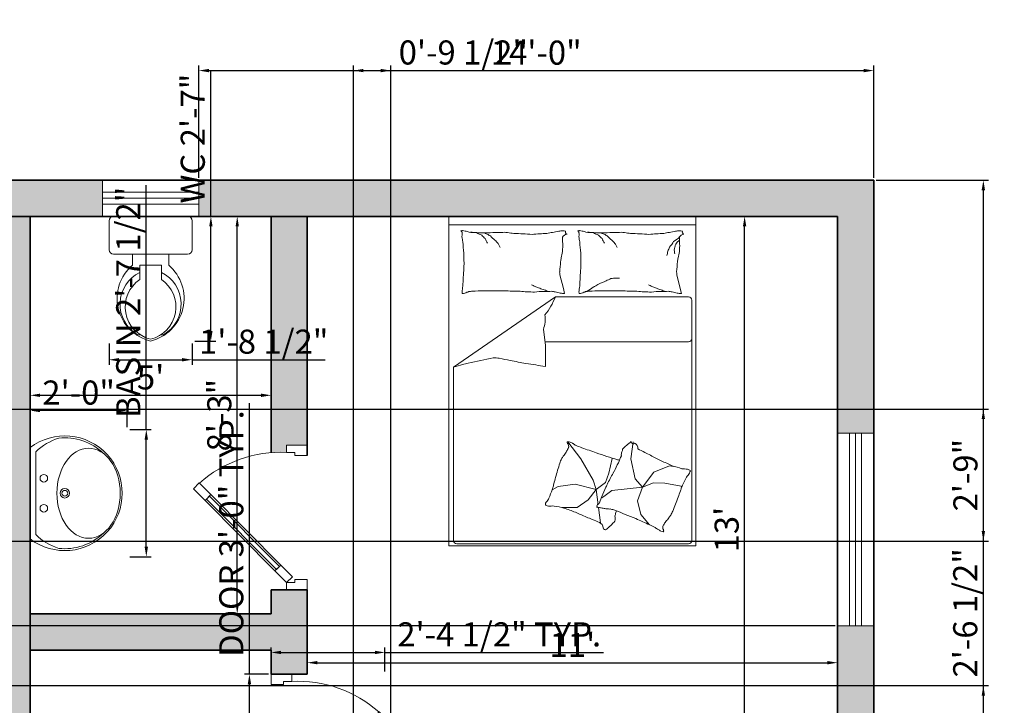
# Model space of a CAD drawing. Units: inches. Extents: x -40 to 424, y -33 to 568.
# Tile 8 of 8: x 171 to 417, y 397 to 568. Entities that reach past the tile are written whole.
import ezdxf

# ---------------------------------------------------------------- set-up
doc = ezdxf.new("R2010")
doc.units = ezdxf.units.IN
for name, color, linetype, lineweight in [('A-ANNO-DIMS', 7, 'Continuous', 18), ('A-DOOR', 7, 'Continuous', 18), ('A-FLOR-FIXT', 7, 'Continuous', 18), ('A-FURN', 7, 'Continuous', 18), ('A-GLAZ', 7, 'Continuous', 18), ('A-WALL-PATT', 30, 'Continuous', 13), ('wall', 7, 'Continuous', 35)]:
    doc.layers.add(name, color=color, linetype=linetype, lineweight=lineweight)
doc.styles.add('DIM_FONT', font='SIMPLEX.shx', dxfattribs={"width": 0.8})
doc.styles.get("Standard").update_dxf_attribs({"font": 'arial.ttf'})
doc.dimstyles.new('ISO-25', dxfattribs={"dimtxt": 6, "dimasz": 2.5, "dimexe": 1.25, "dimexo": 0.625, "dimtad": 1, "dimdec": 1, "dimlunit": 3, "dimtxsty": 'Standard', "dimcen": 2.5, "dimadec": 0, "dimazin": 0, "dimtfac": 1, "dimtdec": 1, "dimtmove": 0, "dimatfit": 3, "dimfxl": 1, "dimarcsym": 0})

# ---------------------------------------------------------------- blocks, each defined once
blk = doc.blocks.new('A$C3C032968')
for p, q in [((0, 0), (0, 100)), ((0, 100), (0, 0)), ((700, 0), (700, 100)), ((700, 0), (700, 100))]:
    blk.add_line(p, q)
for points in [[(517.5, 522.4), (460.7, 466.1), (432.5, 494.5), (489.3, 550.8)], [(120, 128), (460.7, 466.1), (432.5, 494.5), (91.8, 156.4)], [(112.9, 135.1), (453.6, 473.2), (439.5, 487.4), (98.8, 149.3)], [(63.2, 71.6), (120, 128), (91.8, 156.4), (35, 100)], [(35, 100), (0, 100), (0, 0), (50, 0), (50, 50), (50, 60), (35, 60)], [(665, 100), (665, 60), (650, 60), (650, 50), (650, 0), (700, 0), (700, 100)]]:
    blk.add_lwpolyline(points, close=True)
blk.add_arc((72.4, 128.7), 593.3, 357.2313, 41.4937)
blk = doc.blocks.new('A$C79B528CE')
for p, q in [((1.5, 2), (0, 2)), ((0, 2), (0, 0)), ((1.5, 0), (1.5, 2)), ((1.5, 1.9476), (0, 1.9476)), ((0.6954, 1.5617), (0.6748, 1.6443)), ((1.4047, 1.5617), (1.384, 1.6443)), ((0.7029, 1.5317), (0.6954, 1.5617)), ((1.4122, 1.5317), (1.4047, 1.5617)), ((0.6465, 1.5115), (0.0284, 1.0841)), ((0.6465, 1.5115), (1.4542, 1.5115)), ((1.4742, 1.4915), (1.4742, 0.0322)), ((0.574, 1.3138), (0.5876, 1.2184)), ((1.4542, 1.2389), (0.5847, 1.2389)), ((0.5876, 1.2184), (0.5859, 1.0883)), ((0.0284, 0.0322), (0.0284, 1.0841)), ((0.7224, 0.6316), (0.8016, 0.5276)), ((1.119, 0.6317), (1.1052, 0.5286)), ((0.8016, 0.5276), (0.8767, 0.3973)), ((0.9716, 0.4407), (0.9914, 0.5296)), ((1.1052, 0.5286), (1.131, 0.4065)), ((1.2446, 0.4478), (1.3392, 0.4856)), ((1.3392, 0.4856), (1.3632, 0.4822)), ((0.9518, 0.3834), (0.9716, 0.4407)), ((1.1757, 0.355), (1.2446, 0.4478)), ((0.6632, 0.3597), (0.6272, 0.3397)), ((0.766, 0.3736), (0.6632, 0.3597)), ((0.8945, 0.342), (0.766, 0.3736)), ((0.8767, 0.3973), (0.8945, 0.342)), ((0.8945, 0.342), (0.9518, 0.3834)), ((1.131, 0.4065), (1.1757, 0.355)), ((1.1757, 0.355), (1.2428, 0.3825)), ((1.2428, 0.3825), (1.3116, 0.379)), ((1.3116, 0.379), (1.4097, 0.3619)), ((1.4097, 0.3619), (1.413, 0.3554)), ((0.8945, 0.342), (0.8451, 0.2787)), ((0.8945, 0.342), (0.9063, 0.2478)), ((0.9297, 0.2995), (0.9119, 0.256)), ((0.9401, 0.3), (0.928, 0.2914)), ((0.9527, 0.3558), (0.9297, 0.2995)), ((0.99, 0.3361), (0.9401, 0.3)), ((1.1757, 0.355), (0.99, 0.3361)), ((1.1757, 0.355), (1.1448, 0.2725)), ((0.8451, 0.2787), (0.7799, 0.2313)), ((1.1448, 0.2725), (1.1654, 0.19)), ((0.7799, 0.2313), (0.687, 0.2313)), ((0.9081, 0.2331), (0.92, 0.1385)), ((1.1654, 0.19), (1.219, 0.1274)), ((1.4542, 0.0122), (0.0484, 0.0122)), ((0, 0), (1.5, 0))]:
    blk.add_line(p, q)
for centre, radius, start, end in [((0.0726, 1.9139), 0.00342, 291.7883, 340.43603), ((0.0739, 1.9378), 0.0251, 274.30254, 291.7883), ((0.098, 1.9393), 0.0289, 239.34875, 274.30254), ((0.6672, 2.0719), 0.1611, 270, 278.43719), ((0.7086, 2.0011), 0.0904, 258.72762, 270), ((0.7818, 1.9139), 0.00342, 291.7883, 340.43603), ((0.7831, 1.9378), 0.0251, 274.30254, 291.7883), ((0.8072, 1.9393), 0.0289, 239.34875, 274.30254), ((1.3765, 2.0719), 0.1611, 270, 278.43719), ((1.4178, 2.0011), 0.0904, 258.72762, 270), ((0.0743, 1.9085), 0.00232, 340.43603, 101.89306), ((0.0805, 1.9093), 0.00428, 201.9904, 281.89306), ((0.049, 1.8889), 0.0328, 338.57902, 8.13348), ((-0.1611, 1.8253), 0.246, 8.13348, 12.10946), ((0.0959, 1.8994), 0.0156, 158.57902, 201.9904), ((0.279, 1.8867), 0.1983, 187.6809, 192.10946), ((0.0952, 1.8568), 0.0539, 59.34875, 84.74081), ((0.0953, 1.0829), 0.8208, 84.74081, 88.09211), ((0.1612, 2.0005), 0.0992, 254.06476, 274.21588), ((0.2269, 1.9817), 0.0992, 233.91364, 254.06476), ((0.1856, 0.406), 1.4943, 88.09211, 90.57574), ((0.2797, 1.9449), 0.0992, 216.17665, 233.91364), ((0.323, 2.1075), 0.234, 242.76041, 249.13972), ((0.3154, 1.8961), 0.0992, 198.43965, 216.17665), ((0.3084, 1.0293), 0.8732, 90.57574, 94.80185), ((0.2874, 1.949), 0.0768, 231.61143, 242.76041), ((0.5234, 2.1633), 0.3916, 226.18849, 231.61143), ((0.4551, 1.9982), 0.2252, 219.03494, 226.18849), ((0.3125, 2.1919), 0.2897, 267.46141, 274.80185), ((0.3637, 2.0532), 0.1524, 259.81012, 267.46141), ((0.3008, 1.3747), 0.5293, 79.81012, 83.9133), ((0.3945, 0.8466), 1.049, 83.9133, 90), ((0.5954, 1.2129), 0.6827, 90, 97.54685), ((0.6611, 1.6625), 0.2422, 97.54685, 105.74398), ((0.5846, 2.2041), 0.3048, 278.43719, 285.74398), ((0.7204, 1.8579), 0.0342, 94.40021, 153.41948), ((1.1818, 1.8735), 0.4918, 180, 186.23236), ((0.7203, 1.9049), 0.0131, 153.41948, 258.72762), ((0.7836, 1.9085), 0.00232, 340.43603, 101.89306), ((0.7897, 1.9093), 0.00428, 201.9904, 281.89306), ((0.7582, 1.8889), 0.0328, 338.57902, 8.13348), ((0.5482, 1.8253), 0.246, 8.13348, 12.10946), ((0.8051, 1.8994), 0.0156, 158.57902, 201.9904), ((0.9883, 1.8867), 0.1983, 187.6809, 192.10946), ((0.8044, 1.8568), 0.0539, 59.34875, 84.74081), ((0.8046, 1.0829), 0.8208, 84.74081, 88.09211), ((0.8704, 2.0005), 0.0992, 254.06476, 274.21588), ((0.9361, 1.9817), 0.0992, 233.91364, 254.06476), ((0.8948, 0.406), 1.4943, 88.09211, 90.57574), ((0.989, 1.9449), 0.0992, 216.17665, 233.91364), ((1.0323, 2.1075), 0.234, 242.76041, 249.13972), ((1.0247, 1.8961), 0.0992, 198.43965, 216.17665), ((1.0177, 1.0293), 0.8732, 90.57574, 94.80185), ((0.9966, 1.949), 0.0768, 231.61143, 242.76041), ((1.2326, 2.1633), 0.3916, 226.18849, 231.61143), ((1.1643, 1.9982), 0.2252, 219.03494, 226.18849), ((1.0217, 2.1919), 0.2897, 267.46141, 274.80185), ((1.0729, 2.0532), 0.1524, 259.81012, 267.46141), ((1.0101, 1.3747), 0.5293, 79.81012, 83.9133), ((1.1037, 0.8466), 1.049, 83.9133, 90), ((1.3046, 1.2129), 0.6827, 90, 97.54685), ((1.3703, 1.6625), 0.2422, 97.54685, 105.74398), ((1.2938, 2.2041), 0.3048, 278.43719, 285.74398), ((1.3004, 1.9723), 0.1399, 297.20359, 314.90238), ((1.3333, 1.9167), 0.0899, 306.26407, 318.55709), ((1.4296, 1.8579), 0.0342, 94.40021, 153.41948), ((1.891, 1.8735), 0.4918, 180, 186.23236), ((1.4295, 1.9049), 0.0131, 153.41948, 258.72762), ((0.9966, 1.8987), 0.9131, 183.36875, 187.6809), ((0.3426, 1.8591), 0.0493, 208.31676, 219.03494), ((0.4886, 1.9062), 0.2002, 203.00277, 208.31676), ((0.8939, 1.7858), 0.204, 170.31563, 180), ((1.7058, 1.8987), 0.9131, 183.36875, 187.6809), ((1.0518, 1.8591), 0.0493, 208.31676, 219.03494), ((1.1978, 1.9062), 0.2002, 203.00277, 208.31676), ((1.2048, 1.8529), 0.1399, 332.60117, 343.48502), ((1.2401, 1.9123), 0.1399, 314.90238, 332.60117), ((1.3147, 1.8132), 0.0562, 341.2201, 0), ((1.2793, 1.7719), 0.0915, 0, 14.68511), ((1.18, 1.8895), 0.2056, 338.18508, 341.2201), ((1.2381, 1.8881), 0.1511, 334.64488, 338.18508), ((1.3389, 1.8667), 0.0526, 318.55709, 334.64488), ((1.6031, 1.7858), 0.204, 170.31563, 180), ((0.7702, 1.7573), 0.6787, 178.36691, 183.36875), ((0.3686, 1.792), 0.3171, 347.80162, 351.99495), ((1.552, 1.5994), 0.882, 167.80162, 170.31563), ((1.4794, 1.7573), 0.6787, 178.36691, 183.36875), ((1.1897, 1.8023), 0.1399, 343.48502, 354.36887), ((1.0778, 1.792), 0.3171, 347.80162, 351.99495), ((2.2613, 1.5994), 0.882, 167.80162, 170.31563), ((13.7013, 0.85), 13.6356, 176.49514, 176.94504), ((1.4559, 1.6447), 1.3652, 176.94504, 178.36691), ((0.0204, 1.7556), 0.6588, 351.99495, 357.33512), ((14.4105, 0.85), 13.6356, 176.49514, 176.94504), ((2.1651, 1.6447), 1.3652, 176.94504, 178.36691), ((0.7297, 1.7556), 0.6588, 351.99495, 357.33512), ((0.6071, 1.6474), 0.0677, 357.33512, 14.04519), ((0.7753, 2.0834), 0.5066, 290.67428, 294.32653), ((0.9799, 1.6796), 0.058, 274.08277, 290.67428), ((1.0172, 1.8969), 0.2721, 266.4448, 274.08277), ((1.3164, 1.6474), 0.0677, 357.33512, 14.04519), ((0.4014, 1.5209), 0.3212, 170.00164, 176.49514), ((0.2076, 0.9067), 0.7387, 64.68893, 66.51559), ((0.2508, 0.888), 0.7387, 66.51559, 68.34226), ((0.2995, 0.8688), 0.7387, 68.34226, 70.57202), ((0.3537, 0.8497), 0.7387, 70.57202, 72.80178), ((1.1107, 1.5209), 0.3212, 170.00164, 176.49514), ((0.4519, 2.1618), 0.7286, 302.13498, 305.82629), ((0.7388, 1.8508), 0.3126, 296.49848, 302.13498), ((0.3151, 2.8912), 1.4323, 294.32653, 296.49848), ((0.9169, 0.9067), 0.7387, 64.68893, 66.51559), ((0.9601, 0.888), 0.7387, 66.51559, 68.34226), ((1.0087, 0.8688), 0.7387, 68.34226, 70.57202), ((1.0629, 0.8497), 0.7387, 70.57202, 72.80178), ((0.0623, 1.535), 0.0193, 350.00164, 16.69777), ((0.0815, 1.5304), 0.00132, 16.69777, 97.12039), ((0.1072, 1.4467), 0.0875, 97.12039, 106.22115), ((0.1315, 1.4654), 0.0767, 106.22115, 117.28412), ((0.1, 1.5832), 0.0453, 282.86904, 297.28412), ((0.1117, 1.6885), 0.1459, 273.57397, 282.86904), ((0.1384, 2.7103), 1.164, 270.28654, 273.57397), ((0.3078, 7.2662), 5.7185, 269.02962, 270.28654), ((0.4895, 4.9065), 3.3622, 267.39037, 269.02962), ((0.5304, 2.7573), 1.2165, 265.38242, 267.39037), ((0.4077, 0.139), 1.4048, 85.38242, 87.25094), ((0.5669, 1.3138), 0.2301, 87.25094, 101.55856), ((0.5943, 1.6886), 0.1459, 263.56595, 281.55856), ((0.2944, 1.6407), 0.3751, 320.35546, 339.85116), ((0.6593, 1.6599), 0.1197, 252.61359, 263.56595), ((0.608, 1.3144), 0.2297, 72.61359, 80.5159), ((0.6574, 1.2635), 0.2708, 80.5159, 85.91706), ((0.7029, 1.5308), 0.000917, 85.91706, 194.04494), ((0.7716, 1.535), 0.0193, 350.00164, 16.69777), ((0.7908, 1.5304), 0.00132, 16.69777, 97.12039), ((0.8165, 1.4467), 0.0875, 97.12039, 106.22115), ((0.8408, 1.4654), 0.0767, 106.22115, 117.28412), ((0.8093, 1.5832), 0.0453, 282.86904, 297.28412), ((0.8209, 1.6885), 0.1459, 273.57397, 282.86904), ((0.8476, 2.7103), 1.164, 270.28654, 273.57397), ((1.017, 7.2662), 5.7185, 269.02962, 270.28654), ((1.1987, 4.9065), 3.3622, 267.39037, 269.02962), ((1.2397, 2.7573), 1.2165, 265.38242, 267.39037), ((1.1169, 0.139), 1.4048, 85.38242, 87.25094), ((1.2761, 1.3138), 0.2301, 87.25094, 101.55856), ((1.3035, 1.6886), 0.1459, 263.56595, 281.55856), ((1.3685, 1.6599), 0.1197, 252.61359, 263.56595), ((1.3172, 1.3144), 0.2297, 72.61359, 80.5159), ((1.3666, 1.2635), 0.2708, 80.5159, 85.91706), ((1.4121, 1.5308), 0.000917, 85.91706, 194.04494), ((1.4542, 1.4915), 0.02, 0, 90), ((0.4049, 1.3759), 0.1801, 339.85116, 8.13558), ((1.4542, 1.2589), 0.02, 270, 0), ((-0.6395, 5.1029), 4.0646, 280.72756, 282.92554), ((0.2775, 1.1989), 0.0581, 262.26962, 280.72756), ((0.3326, 1.3309), 0.1942, 256.8096, 262.26962), ((-0.2025, -1.3253), 2.5158, 76.8096, 78.32586), ((-0.4754, 2.8487), 1.8351, 285.93519, 287.73639), ((-0.0634, 1.7415), 0.6574, 282.92554, 285.93519), ((-0.0554, -1.4284), 2.588, 78.32586, 80.50498), ((-0.0377, -2.64), 3.7801, 80.50498, 82.308), ((0.7246, 0.6267), 0.0063, 166.71916, 233.42082), ((0.7227, 0.6272), 0.00443, 93.94836, 166.71916), ((0.7124, 0.6103), 0.0142, 10.40739, 53.42082), ((0.7249, 0.5964), 0.0352, 69.65479, 93.94836), ((0.6889, 0.6079), 0.0393, 333.18207, 345.42909), ((0.6504, 0.5989), 0.0771, 2.72862, 10.40739), ((0.7122, 0.6019), 0.0153, 345.42909, 2.72862), ((0.7162, 0.5731), 0.0601, 51.41461, 69.65479), ((0.8031, 0.682), 0.0792, 231.41461, 247.29308), ((1.0957, 1.3811), 0.8371, 247.29308, 249.87133), ((0.9323, 0.7705), 0.2176, 307.21509, 313.52244), ((0.692, 1.1456), 0.6605, 306.2163, 307.21509), ((1.3244, 0.3162), 0.3825, 126.2163, 127.52874), ((1.1299, 0.5924), 0.0452, 127.52874, 134.1274), ((1.0587, 0.6825), 0.0697, 308.81361, 314.1274), ((1.1199, 0.6318), 0.0127, 176.75451, 308.81361), ((1.1115, 0.59), 0.0359, 356.75451, 62.70976), ((0.7571, 0.4922), 0.081, 140.29953, 153.92651), ((0.5455, 0.6678), 0.194, 320.29953, 329.09437), ((0.4099, 0.749), 0.352, 329.09437, 333.18207), ((2.5607, 5.3783), 5.0942, 249.87133, 250.91638), ((1.9234, 3.5362), 3.145, 250.91638, 253.39153), ((1.9583, 0.1204), 1.0054, 154.94715, 157.58378), ((1.0928, 0.5526), 0.0458, 157.58378, 188.04918), ((1.0322, 0.5833), 0.0226, 324.10643, 8.04918), ((1.0012, 0.6426), 0.0774, 313.52244, 324.10643), ((-0.2306, -2.1858), 3.0972, 62.70976, 63.58535), ((2.1205, 2.3551), 2.0162, 242.50014, 243.58535), ((4.0739, 5.9445), 6.1019, 242.15178, 242.50014), ((2.5804, -0.112), 2.003, 162.1604, 164.73746), ((0.8608, 0.4414), 0.1965, 153.92651, 162.1604), ((2.5307, -0.2643), 1.6868, 152.91165, 154.94715), ((1.0578, 0.6341), 0.1166, 253.39153, 259.26338), ((-1.4387, -4.647), 5.8383, 62.15178, 62.50792), ((1.0676, -0.068), 0.6236, 62.50792, 69.25137), ((1.2615, 0.0657), 0.43, 69.25137, 77.37478), ((2.3589, -0.3311), 1.5652, 150.06403, 152.91165), ((1.4175, 0.4049), 0.063, 77.37478, 93.38812), ((1.4448, 0.5247), 0.0599, 256.95977, 273.38812), ((1.3928, 0.4743), 0.0755, 310.50865, 333.66682), ((1.4751, 0.5082), 0.0509, 238.30826, 256.95977), ((1.4772, 0.441), 0.0168, 130.50865, 180.96136), ((1.4694, 0.4587), 0.0058, 180.96136, 238.30826), ((0.1082, 0.5062), 0.5454, 343.68776, 346.159), ((2.2381, -0.0186), 1.6481, 164.73746, 166.159), ((0.767, 0.4627), 0.2143, 330.06403, 337.76452), ((1.2503, 0.4319), 0.1798, 334.82685, 339.29188), ((-0.9672, 1.5491), 2.6619, 333.66682, 334.82685), ((-1.8615, 1.284), 2.6619, 338.0627, 339.22273), ((0.4592, 0.4035), 0.1798, 339.22273, 343.68776), ((2.9572, -0.2212), 1.6481, 160.34158, 161.76311), ((0.895, 0.5261), 0.5454, 339.29188, 341.76311), ((0.6027, 0.2524), 0.0168, 134.90453, 185.35724), ((0.5918, 0.2513), 0.0058, 185.35724, 242.70414), ((0.6125, 0.2914), 0.0509, 242.70414, 261.35565), ((0.5376, 0.3177), 0.0755, 314.90453, 338.0627), ((0.6138, 0.3003), 0.0599, 261.35565, 277.784), ((0.6305, 0.1786), 0.063, 81.77066, 97.784), ((0.5779, -0.1846), 0.43, 73.64725, 81.77066), ((0.8959, 0.2383), 0.00467, 287.18674, 70.62007), ((0.9188, 0.234), 0.0231, 107.18674, 157.76452), ((3.2459, -0.4634), 2.003, 157.76452, 160.34158), ((0.5234, -0.3705), 0.6236, 66.9038, 73.64725), ((-1.5222, -5.1672), 5.8383, 66.54766, 66.9038), ((3.2298, 5.7866), 6.1019, 246.54766, 246.89602), ((0.8979, 0.2247), 0.0092, 70.62007, 94.25932), ((0.9057, 0.267), 0.034, 262.01776, 274.25932), ((0.9584, 0.4221), 0.1955, 255.1193, 262.01776), ((0.9073, 0.0507), 0.1794, 75.1193, 82.32164), ((0.959, 0.153), 0.0712, 82.32164, 94.51184), ((0.9779, 0.2893), 0.0663, 261.87843, 274.51184), ((1.0249, 0.332), 0.1166, 248.99565, 261.87843), ((2.2614, 3.1012), 3.145, 246.5205, 248.99565), ((1.0543, 0.1766), 0.0458, 161.97966, 192.44506), ((1.9669, -0.1202), 1.0054, 160.65521, 161.97966), ((1.4053, 0.1288), 0.081, 135.90365, 149.53063), ((1.529, 0.1108), 0.1965, 149.53063, 157.76452), ((1.6266, 2.0287), 2.0162, 246.89602, 247.98123), ((-0.2904, -2.7118), 3.0972, 67.10564, 67.98123), ((0.9005, 0.1084), 0.0359, 1.15039, 67.10564), ((0.5426, 0.6156), 0.6605, 310.61218, 311.61098), ((0.8367, 0.2845), 0.2176, 311.61098, 317.91833), ((0.9408, 0.1905), 0.0774, 317.91833, 328.50231), ((0.9875, 0.1619), 0.0226, 328.50231, 12.44506), ((3.2487, 4.7998), 5.0942, 245.47545, 246.5205), ((1.6004, 0.8725), 0.8371, 242.8972, 245.47545), ((1.2655, 0.1388), 0.0393, 328.78619, 341.03321), ((1.0155, 0.3294), 0.352, 324.69849, 328.78619), ((1.1772, 0.2819), 0.194, 315.90365, 324.69849), ((0.9491, 0.1094), 0.0127, 181.15039, 313.2095), ((0.9101, 0.1509), 0.0697, 313.2095, 318.52329), ((0.9962, 0.0748), 0.0452, 131.92462, 138.52329), ((1.2216, -0.1762), 0.3825, 130.61218, 131.92462), ((1.3069, 0.1689), 0.0792, 227.01873, 242.8972), ((1.2457, 0.0438), 0.0601, 47.01873, 65.25891), ((1.2864, 0.0526), 0.0352, 65.25891, 89.55248), ((1.2839, 0.1188), 0.0153, 341.03321, 358.33274), ((1.2216, 0.1058), 0.0771, 358.33274, 6.01151), ((1.2895, 0.0928), 0.0142, 6.01151, 49.02494), ((1.3054, 0.0832), 0.00443, 89.55248, 162.32327), ((1.3095, 0.0924), 0.0063, 162.32327, 229.02494), ((0.0484, 0.0322), 0.02, 180, 270), ((1.4542, 0.0322), 0.02, 270, 0)]:
    blk.add_arc(centre, radius, start, end)
at = {"style": 'DIM_FONT', "oblique": -180, "text_generation_flag": 4, "width": 0.8, "flags": 9}
for tag in ['XSIZE', 'YSIZE']:
    blk.add_attdef(tag, (1.5, 2), '', height=0.0005, rotation=180, dxfattribs=at)
blk = doc.blocks.new('A$C178D0859')
for p, q in [((0.06, 0.4825), (0.5383, 0.4825)), ((0.0823, 0.4525), (0.516, 0.4525))]:
    blk.add_line(p, q)
at = {"ltscale": 0.06}
for centre in [(0.2205, 0.4103), (0.3778, 0.4103)]:
    blk.add_circle(centre, 0.02, dxfattribs=at)
for radius in [0.025, 0.015]:
    blk.add_circle((0.2991, 0.3005), radius)
for centre, radius, start, end in [((0.2991, 0.3005), 0.3005, 142.7238, 37.2762), ((0.2991, 0.2413), 0.3027, 135.7485, 162.5332), ((0.2991, 0.2413), 0.3027, 17.4668, 44.2515), ((0.2991, 0.3005), 0.2905, 173.7519, 224.0266), ((0.2991, 0.3005), 0.2905, 315.9734, 6.2481)]:
    blk.add_arc(centre, radius, start, end)
blk.add_ellipse((0.2991, 0.176), major_axis=(-0.2361, 0), ratio=0.703116)
blk = doc.blocks.new('A$C02F3725D')
for p, q in [((0, 0.505), (0, 0.665)), ((0.025, 0.69), (0.435, 0.69)), ((0.46, 0.665), (0.46, 0.505)), ((0.435, 0.48), (0.025, 0.48)), ((0.13, 0.48), (0.13, 0.42)), ((0.33, 0.42), (0.33, 0.48)), ((0.17, 0.34), (0.17, 0.42)), ((0.17, 0.42), (0.29, 0.42)), ((0.29, 0.34), (0.29, 0.42)), ((0.1578, 0.035), (0.1724, 0.035)), ((0.2876, 0.035), (0.3022, 0.035))]:
    blk.add_line(p, q)
for centre, radius, start, end in [((0.025, 0.665), 0.025, 90, 180), ((0.435, 0.665), 0.025, 0, 90), ((0.025, 0.505), 0.025, 180, 270), ((0.435, 0.505), 0.025, 270, 0), ((0.2874, 0.2356), 0.2425, 130.4885, 256.2965), ((0.1726, 0.2356), 0.2425, 283.7035, 49.5115), ((0.2568, 0.2042), 0.196, 116.2742, 239.6668), ((0.2732, 0.1883), 0.1834, 124.2157, 256.394), ((0.1868, 0.1883), 0.1834, 283.606, 55.7843), ((0.2032, 0.2042), 0.196, 300.3332, 63.7258)]:
    blk.add_arc(centre, radius, start, end)
blk = doc.blocks.new('*D31')
at = {"layer": 'A-ANNO-DIMS', "color": 0, "lineweight": -2, "transparency": 16777216}
for p, q in [((174, 483.07), (174, 473.19)), ((234, 483.07), (234, 473.19)), ((176.5, 474.44), (231.5, 474.44))]:
    blk.add_line(p, q, dxfattribs=at)
at = {"layer": 'A-ANNO-DIMS', "color": 0, "transparency": 16777216}
for points in [[(176.5, 474.85), (176.5, 474.02), (174, 474.44)], [(231.5, 474.85), (231.5, 474.02), (234, 474.44)]]:
    blk.add_solid(points, dxfattribs=at)
at = {"layer": 'Defpoints', "color": 0, "transparency": 16777216}
for p in [(174, 483.69), (234, 483.69), (234, 474.44)]:
    blk.add_point(p, dxfattribs=at)
at = {"layer": 'A-ANNO-DIMS', "color": 0, "transparency": 16777216, "insert": (204, 478.11), "char_height": 6, "attachment_point": 5}
blk.add_mtext("5'", dxfattribs=at)
blk = doc.blocks.new('*D32')
at = {"layer": 'A-ANNO-DIMS', "color": 0, "lineweight": -2, "transparency": 16777216}
for p, q in [((226.2, 519), (226.82, 519)), ((225.57, 422.5), (225.57, 516.5)), ((204.63, 420), (226.82, 420))]:
    blk.add_line(p, q, dxfattribs=at)
at = {"layer": 'A-ANNO-DIMS', "color": 0, "transparency": 16777216}
for points in [[(225.16, 516.5), (225.99, 516.5), (225.57, 519)], [(225.16, 422.5), (225.99, 422.5), (225.57, 420)]]:
    blk.add_solid(points, dxfattribs=at)
at = {"layer": 'Defpoints', "color": 0, "transparency": 16777216}
for p in [(225.57, 519), (225.57, 519), (204, 420)]:
    blk.add_point(p, dxfattribs=at)
at = {"layer": 'A-ANNO-DIMS', "color": 0, "transparency": 16777216, "insert": (221.88, 469.5), "char_height": 6, "attachment_point": 5, "rotation": 90}
blk.add_mtext('8\'-3"', dxfattribs=at)
blk = doc.blocks.new('*D33')
at = {"layer": 'A-ANNO-DIMS', "color": 0, "lineweight": -2, "transparency": 16777216}
for p, q in [((243, 414.87), (243, 406.6)), ((375, 416.38), (375, 406.6)), ((245.5, 407.85), (372.5, 407.85))]:
    blk.add_line(p, q, dxfattribs=at)
at = {"layer": 'A-ANNO-DIMS', "color": 0, "transparency": 16777216}
for points in [[(245.5, 408.27), (245.5, 407.44), (243, 407.85)], [(372.5, 408.27), (372.5, 407.44), (375, 407.85)]]:
    blk.add_solid(points, dxfattribs=at)
at = {"layer": 'Defpoints', "color": 0, "transparency": 16777216}
for p in [(375, 417), (243, 415.5), (375, 407.85)]:
    blk.add_point(p, dxfattribs=at)
at = {"layer": 'A-ANNO-DIMS', "color": 0, "transparency": 16777216, "insert": (309, 411.49), "char_height": 6, "attachment_point": 5}
blk.add_mtext("11'", dxfattribs=at)
blk = doc.blocks.new('*D34')
at = {"layer": 'A-ANNO-DIMS', "color": 0, "lineweight": -2, "transparency": 16777216}
for p, q in [((353.15, 519), (350.62, 519)), ((351.87, 365.5), (351.87, 516.5)), ((353.15, 363), (350.62, 363))]:
    blk.add_line(p, q, dxfattribs=at)
at = {"layer": 'A-ANNO-DIMS', "color": 0, "transparency": 16777216}
for points in [[(351.46, 516.5), (352.29, 516.5), (351.87, 519)], [(351.46, 365.5), (352.29, 365.5), (351.87, 363)]]:
    blk.add_solid(points, dxfattribs=at)
at = {"layer": 'Defpoints', "color": 0, "transparency": 16777216}
for p in [(351.87, 519), (353.78, 519), (353.78, 363)]:
    blk.add_point(p, dxfattribs=at)
at = {"layer": 'A-ANNO-DIMS', "color": 0, "transparency": 16777216, "insert": (348.18, 441), "char_height": 6, "attachment_point": 5, "rotation": 90}
blk.add_mtext("13'", dxfattribs=at)
blk = doc.blocks.new('WIN-48IN')
for p, q in [((0, 0), (0, 9)), ((48, 0), (48, 9)), ((0, 6), (48, 6)), ((0, 4.5), (48, 4.5)), ((0, 3), (48, 3))]:
    blk.add_line(p, q)
blk = doc.blocks.new('WIN-24IN')
for p, q in [((9, 24), (0, 24)), ((3, 0), (3, 24)), ((4.5, 0), (4.5, 24)), ((6, 0), (6, 24)), ((9, 0), (0, 0))]:
    blk.add_line(p, q)
blk = doc.blocks.new('*D47')
at = {"layer": 'A-ANNO-DIMS', "color": 0, "lineweight": -2, "transparency": 16777216}
for p, q in [((228.6, 405), (228.6, 472.5)), ((233.37, 405), (227.35, 405)), ((228.6, 371.5), (228.6, 402.5)), ((233.37, 369), (227.35, 369))]:
    blk.add_line(p, q, dxfattribs=at)
at = {"layer": 'A-ANNO-DIMS', "color": 0, "transparency": 16777216}
for points in [[(228.18, 402.5), (229.02, 402.5), (228.6, 405)], [(228.18, 371.5), (229.02, 371.5), (228.6, 369)]]:
    blk.add_solid(points, dxfattribs=at)
at = {"layer": 'Defpoints', "color": 0, "transparency": 16777216}
for p in [(228.6, 405), (234, 405), (234, 369)]:
    blk.add_point(p, dxfattribs=at)
at = {"layer": 'A-ANNO-DIMS', "color": 0, "transparency": 16777216, "insert": (224.87, 440), "char_height": 6, "attachment_point": 5, "rotation": 90}
blk.add_mtext('DOOR 3\'-0" TYP.', dxfattribs=at)
blk = doc.blocks.new('*D48')
at = {"layer": 'A-ANNO-DIMS', "color": 0, "lineweight": -2, "transparency": 16777216}
for p, q in [((234, 405.63), (234, 411.65)), ((236.5, 410.4), (259.83, 410.4)), ((262.33, 405.63), (262.33, 411.65)), ((262.33, 410.4), (316.73, 410.4))]:
    blk.add_line(p, q, dxfattribs=at)
at = {"layer": 'A-ANNO-DIMS', "color": 0, "transparency": 16777216}
for points in [[(236.5, 410.82), (236.5, 409.98), (234, 410.4)], [(259.83, 410.82), (259.83, 409.98), (262.33, 410.4)]]:
    blk.add_solid(points, dxfattribs=at)
at = {"layer": 'Defpoints', "color": 0, "transparency": 16777216}
for p in [(262.33, 410.4), (234, 405), (262.33, 405)]:
    blk.add_point(p, dxfattribs=at)
at = {"layer": 'A-ANNO-DIMS', "color": 0, "transparency": 16777216, "insert": (290.78, 414.13), "char_height": 6, "attachment_point": 5}
blk.add_mtext('2\'-4 1/2" TYP.', dxfattribs=at)
blk = doc.blocks.new('*D63')
at = {"layer": 'A-ANNO-DIMS', "color": 0, "lineweight": -2, "transparency": 16777216}
for p, q in [((202.93, 465.9), (202.93, 526.79)), ((198.81, 465.9), (204.18, 465.9)), ((202.93, 436.71), (202.93, 463.4)), ((198.81, 434.21), (204.18, 434.21))]:
    blk.add_line(p, q, dxfattribs=at)
at = {"layer": 'A-ANNO-DIMS', "color": 0, "transparency": 16777216}
for points in [[(202.52, 463.4), (203.35, 463.4), (202.93, 465.9)], [(202.52, 436.71), (203.35, 436.71), (202.93, 434.21)]]:
    blk.add_solid(points, dxfattribs=at)
at = {"layer": 'Defpoints', "color": 0, "transparency": 16777216}
for p in [(198.18, 465.9), (202.93, 465.9), (198.18, 434.21)]:
    blk.add_point(p, dxfattribs=at)
at = {"layer": 'A-ANNO-DIMS', "color": 0, "transparency": 16777216, "insert": (199.21, 497.59), "char_height": 6, "attachment_point": 5, "rotation": 90}
blk.add_mtext('BASIN 2\'-7 1/2"', dxfattribs=at)
blk = doc.blocks.new('*D64')
at = {"layer": 'A-ANNO-DIMS', "color": 0, "lineweight": -2, "transparency": 16777216}
for p, q in [((174, 466.52), (174, 471.9)), ((195.68, 470.65), (176.5, 470.65)), ((198.18, 466.52), (198.18, 471.9))]:
    blk.add_line(p, q, dxfattribs=at)
at = {"layer": 'A-ANNO-DIMS', "color": 0, "transparency": 16777216}
for points in [[(176.5, 471.07), (176.5, 470.23), (174, 470.65)], [(195.68, 471.07), (195.68, 470.23), (198.18, 470.65)]]:
    blk.add_solid(points, dxfattribs=at)
at = {"layer": 'Defpoints', "color": 0, "transparency": 16777216}
for p in [(174, 470.65), (174, 465.9), (198.18, 465.9)]:
    blk.add_point(p, dxfattribs=at)
at = {"layer": 'A-ANNO-DIMS', "color": 0, "transparency": 16777216, "insert": (186.09, 474.34), "char_height": 6, "attachment_point": 5}
blk.add_mtext('2\'-0"', dxfattribs=at)
blk = doc.blocks.new('*D67')
at = {"layer": 'A-ANNO-DIMS', "color": 0, "lineweight": -2, "transparency": 16777216}
for p, q in [((219.01, 519), (219.01, 555.24)), ((214.98, 519), (220.26, 519)), ((219.01, 490.45), (219.01, 516.5)), ((214.98, 487.95), (220.26, 487.95))]:
    blk.add_line(p, q, dxfattribs=at)
at = {"layer": 'A-ANNO-DIMS', "color": 0, "transparency": 16777216}
for points in [[(218.59, 516.5), (219.43, 516.5), (219.01, 519)], [(218.59, 490.45), (219.43, 490.45), (219.01, 487.95)]]:
    blk.add_solid(points, dxfattribs=at)
at = {"layer": 'Defpoints', "color": 0, "transparency": 16777216}
for p in [(214.35, 519), (219.01, 519), (214.35, 487.95)]:
    blk.add_point(p, dxfattribs=at)
at = {"layer": 'A-ANNO-DIMS', "color": 0, "transparency": 16777216, "insert": (215.28, 538.37), "char_height": 6, "attachment_point": 5, "rotation": 90}
blk.add_mtext('WC 2\'-7"', dxfattribs=at)
blk = doc.blocks.new('*D68')
at = {"layer": 'A-ANNO-DIMS', "color": 0, "lineweight": -2, "transparency": 16777216}
for p, q in [((193.65, 487.32), (193.65, 482.04)), ((214.35, 487.32), (214.35, 482.04)), ((196.15, 483.29), (211.85, 483.29)), ((214.35, 483.29), (247.47, 483.29))]:
    blk.add_line(p, q, dxfattribs=at)
at = {"layer": 'A-ANNO-DIMS', "color": 0, "transparency": 16777216}
for points in [[(196.15, 483.71), (196.15, 482.87), (193.65, 483.29)], [(211.85, 483.71), (211.85, 482.87), (214.35, 483.29)]]:
    blk.add_solid(points, dxfattribs=at)
at = {"layer": 'Defpoints', "color": 0, "transparency": 16777216}
for p in [(193.65, 487.95), (214.35, 487.95), (214.35, 483.29)]:
    blk.add_point(p, dxfattribs=at)
at = {"layer": 'A-ANNO-DIMS', "color": 0, "transparency": 16777216, "insert": (232.16, 487.02), "char_height": 6, "attachment_point": 5}
blk.add_mtext('1\'-8 1/2"', dxfattribs=at)
blk = doc.blocks.new('*D80')
at = {"layer": 'A-ANNO-DIMS', "color": 0, "lineweight": -2, "transparency": 16777216}
for p, q in [((384.63, 528), (412.55, 528)), ((411.3, 2.5), (411.3, 525.5)), ((384.63, 0), (412.55, 0))]:
    blk.add_line(p, q, dxfattribs=at)
at = {"layer": 'A-ANNO-DIMS', "color": 0, "transparency": 16777216}
for points in [[(410.88, 525.5), (411.72, 525.5), (411.3, 528)], [(410.88, 2.5), (411.72, 2.5), (411.3, 0)]]:
    blk.add_solid(points, dxfattribs=at)
at = {"layer": 'Defpoints', "color": 0, "transparency": 16777216}
for p in [(384, 528), (411.3, 528), (384, 0)]:
    blk.add_point(p, dxfattribs=at)
at = {"layer": 'A-ANNO-DIMS', "color": 0, "transparency": 16777216, "insert": (407.61, 264), "char_height": 6, "attachment_point": 5, "rotation": 90}
blk.add_mtext('44\'-0"', dxfattribs=at)
blk = doc.blocks.new('*D86')
at = {"layer": 'A-ANNO-DIMS', "color": 0, "lineweight": -2, "transparency": 16777216}
for p, q in [((216, 528.62), (216, 556.55)), ((384, 528.62), (384, 556.55)), ((218.5, 555.3), (381.5, 555.3))]:
    blk.add_line(p, q, dxfattribs=at)
at = {"layer": 'A-ANNO-DIMS', "color": 0, "transparency": 16777216}
for points in [[(218.5, 555.72), (218.5, 554.88), (216, 555.3)], [(381.5, 555.72), (381.5, 554.88), (384, 555.3)]]:
    blk.add_solid(points, dxfattribs=at)
at = {"layer": 'Defpoints', "color": 0, "transparency": 16777216}
for p in [(384, 555.3), (216, 528), (384, 528)]:
    blk.add_point(p, dxfattribs=at)
at = {"layer": 'A-ANNO-DIMS', "color": 0, "transparency": 16777216, "insert": (300, 558.99), "char_height": 6, "attachment_point": 5}
blk.add_mtext('14\'-0"', dxfattribs=at)
blk = doc.blocks.new('*D89')
at = {"layer": 'A-ANNO-DIMS', "color": 0, "lineweight": -2, "transparency": 16777216}
for p, q in [((374.38, 417), (-28.55, 417)), ((-27.3, 365.5), (-27.3, 414.5)), ((374.38, 363), (-28.55, 363))]:
    blk.add_line(p, q, dxfattribs=at)
at = {"layer": 'A-ANNO-DIMS', "color": 0, "transparency": 16777216}
for points in [[(-27.72, 414.5), (-26.88, 414.5), (-27.3, 417)], [(-27.72, 365.5), (-26.88, 365.5), (-27.3, 363)]]:
    blk.add_solid(points, dxfattribs=at)
at = {"layer": 'Defpoints', "color": 0, "transparency": 16777216}
for p in [(-27.3, 417), (375, 417), (375, 363)]:
    blk.add_point(p, dxfattribs=at)
at = {"layer": 'A-ANNO-DIMS', "color": 0, "transparency": 16777216, "insert": (-30.99, 390), "char_height": 6, "attachment_point": 5, "rotation": 90}
blk.add_mtext('4\'-6"', dxfattribs=at)
blk = doc.blocks.new('*D98')
at = {"layer": 'A-ANNO-DIMS', "color": 0, "lineweight": -2, "transparency": 16777216}
for p, q in [((254.5, 312.12), (254.5, 556.55)), ((263.77, 312.12), (263.77, 556.55)), ((257, 555.3), (261.27, 555.3)), ((263.77, 555.3), (297.45, 555.3))]:
    blk.add_line(p, q, dxfattribs=at)
at = {"layer": 'A-ANNO-DIMS', "color": 0, "transparency": 16777216}
for points in [[(257, 555.72), (257, 554.88), (254.5, 555.3)], [(261.27, 555.72), (261.27, 554.88), (263.77, 555.3)]]:
    blk.add_solid(points, dxfattribs=at)
at = {"layer": 'Defpoints', "color": 0, "transparency": 16777216}
for p in [(263.77, 555.3), (254.5, 311.5), (263.77, 311.5)]:
    blk.add_point(p, dxfattribs=at)
at = {"layer": 'A-ANNO-DIMS', "color": 0, "transparency": 16777216, "insert": (281.86, 559.03), "char_height": 6, "attachment_point": 5}
blk.add_mtext('0\'-9 1/2"', dxfattribs=at)
blk = doc.blocks.new('*D102')
at = {"layer": 'A-ANNO-DIMS', "color": 0, "lineweight": -2, "transparency": 16777216}
for p, q in [((29.83, 471), (412.55, 471)), ((411.3, 440.63), (411.3, 468.5)), ((29.83, 438.13), (412.55, 438.13))]:
    blk.add_line(p, q, dxfattribs=at)
at = {"layer": 'A-ANNO-DIMS', "color": 0, "transparency": 16777216}
for points in [[(410.88, 468.5), (411.72, 468.5), (411.3, 471)], [(410.88, 440.63), (411.72, 440.63), (411.3, 438.13)]]:
    blk.add_solid(points, dxfattribs=at)
at = {"layer": 'Defpoints', "color": 0, "transparency": 16777216}
for p in [(29.21, 471), (411.3, 471), (29.21, 438.13)]:
    blk.add_point(p, dxfattribs=at)
at = {"layer": 'A-ANNO-DIMS', "color": 0, "transparency": 16777216, "insert": (407.61, 454.56), "char_height": 6, "attachment_point": 5, "rotation": 90}
blk.add_mtext('2\'-9"', dxfattribs=at)
blk = doc.blocks.new('*D103')
at = {"layer": 'A-ANNO-DIMS', "color": 0, "lineweight": -2, "transparency": 16777216}
for p, q in [((411.3, 402.13), (411.3, 435.91)), ((34.13, 402.13), (412.55, 402.13)), ((411.3, 374.13), (411.3, 399.63)), ((34.13, 371.63), (412.55, 371.63))]:
    blk.add_line(p, q, dxfattribs=at)
at = {"layer": 'A-ANNO-DIMS', "color": 0, "transparency": 16777216}
for points in [[(410.88, 399.63), (411.72, 399.63), (411.3, 402.13)], [(410.88, 374.13), (411.72, 374.13), (411.3, 371.63)]]:
    blk.add_solid(points, dxfattribs=at)
at = {"layer": 'Defpoints', "color": 0, "transparency": 16777216}
for p in [(33.5, 402.13), (411.3, 402.13), (33.5, 371.63)]:
    blk.add_point(p, dxfattribs=at)
at = {"layer": 'A-ANNO-DIMS', "color": 0, "transparency": 16777216, "insert": (407.57, 420.27), "char_height": 6, "attachment_point": 5, "rotation": 90}
blk.add_mtext('2\'-6 1/2"', dxfattribs=at)

msp = doc.modelspace()

# ---------------------------------------------------------------- hatches: boundary and pattern name
at = {"layer": 'A-WALL-PATT'}
h = msp.add_hatch(color=256, dxfattribs=at)
h.dxf.hatch_style = 1
h.paths.add_polyline_path([(9, 399), (0, 399), (0, 351), (9, 351)])
h.paths.add_polyline_path([(9, 303), (0, 303), (0, 210), (9, 210)])
h.paths.add_polyline_path([(9, 150), (0, 150), (0, 0), (384, 0), (384, 69), (375, 69), (375, 62.24), (375, 9), (9, 9)])
h.paths.add_polyline_path([(210, 177), (216, 177), (216, 186), (210, 186), (210, 216), (201, 216), (201, 90), (195, 90), (195, 81), (201, 81), (201, 9), (210, 9)])
h.paths.add_polyline_path([(384, 216), (375, 216), (375, 117), (384, 117)])
h.paths.add_polyline_path([(384, 298.5), (375, 298.5), (375, 279), (375, 240), (384, 240)])
h.paths.add_polyline_path([(384, 417), (375, 417), (375, 334.5), (384, 334.5)])
h.paths.add_polyline_path([(384, 528), (216, 528), (216, 519), (375, 519), (375, 465), (384, 465)])
h.paths.add_polyline_path([(192, 528), (0, 528), (0, 511.5), (9, 511.5), (9, 519), (192, 519)])
h.paths.add_polyline_path([(9, 487.5), (0, 487.5), (0, 447), (9, 447)])
h.paths.add_polyline_path([(111, 480), (9, 480), (9, 471), (111, 471)])
h.paths.add_polyline_path([(174, 519), (165, 519), (165, 354), (174, 354)])
h.paths.add_polyline_path([(243, 426), (237.86, 426), (234, 426), (234, 420), (174, 420), (174, 411), (234, 411), (234, 405), (239.14, 405), (243, 405)])
h.paths.add_polyline_path([(243, 519), (234, 519), (234, 460.14, -0.031638), (237.86, 460.2), (237.86, 462), (243, 462)])
h.paths.add_polyline_path([(243, 369), (234, 369), (234, 354), (375, 354), (375, 363), (243, 363)])
h.paths.add_polyline_path([(375, 279), (195, 279), (195, 270), (201, 270), (201, 264), (210, 264), (210, 270), (375, 270)])
h.paths.add_polyline_path([(291, 270), (282, 270), (282, 222), (286.29, 222), (291, 222)])
h.paths.add_polyline_path([(375, 186), (291, 186), (291, 192), (282, 192), (282, 186), (252, 186), (252, 180.86), (252, 177), (375, 177)])
h.paths.add_polyline_path([(147, 279), (9, 279), (9, 270), (147, 270)])

# ---------------------------------------------------------------- linework, layer by layer
at = {"layer": 'wall'}
for p, q in [((375, 519), (9, 519)), ((174, 519), (174, 354)), ((234, 519), (234, 460.14)), ((243, 519), (243, 459.43)), ((375, 9), (375, 519)), ((243, 426), (234, 426)), ((234, 426), (234, 420)), ((243, 426), (243, 405)), ((234, 420), (174, 420)), ((234, 411), (174, 411)), ((234, 411), (234, 405)), ((243, 405), (234, 405))]:
    msp.add_line(p, q, dxfattribs=at)
msp.add_lwpolyline([(0, 0), (384, 0), (384, 528), (0, 528)], close=True, dxfattribs=at)

# ---------------------------------------------------------------- block references
at = {"layer": 'A-DOOR', "yscale": 0.0514285714285714, "zscale": 0.0514285714285714}
for p, xscale, rotation in [((243, 426), 0.0514285714285714, 90), ((234, 369), -0.0514285714285714, 269.9999999999998)]:
    msp.add_blockref('A$C3C032968', p, dxfattribs=dict(at, xscale=xscale, rotation=rotation))
at = {"layer": 'A-FLOR-FIXT', "xscale": 45.00381884067351, "yscale": 45.00381884067351, "zscale": 45.00381884067351}
msp.add_blockref('A$C02F3725D', (193.65, 487.95), dxfattribs=at)
at = {"layer": 'A-FLOR-FIXT', "xscale": 47.53220188141009, "yscale": 47.53220188141009, "zscale": 47.53220188141009, "rotation": 90}
msp.add_blockref('A$C178D0859', (196.93, 435.83), dxfattribs=at)
at = {"layer": 'A-FURN', "xscale": 41.01472337562348, "yscale": 41.01472337562348, "zscale": 41.01472337562348}
msp.add_blockref('A$C79B528CE', (278.24, 436.97), dxfattribs=at)
at = {"layer": 'A-GLAZ'}
for name, p, rotation in [('WIN-24IN', (216, 519), 90), ('WIN-48IN', (384, 417), 90.00000000000003)]:
    msp.add_blockref(name, p, dxfattribs=dict(at, rotation=rotation))

# ---------------------------------------------------------------- dimensions: what is measured, and where the dimension line sits
at = {"layer": 'A-ANNO-DIMS'}
for base, p1, p2, override, picture, middle in [((263.77, 555.3), (254.5, 311.5), (263.77, 311.5), {"dimdec": 1, "dimlfac": 1, "dimrnd": 0, "dimzin": 1, "dimdsep": 46, "dimlunit": 4, "dimfrac": 2}, '*D98', (281.86, 559.03)), ((384, 555.3), (216, 528), (384, 528), {"dimdec": 1, "dimlfac": 1, "dimrnd": 0, "dimzin": 1, "dimdsep": 46, "dimlunit": 4, "dimfrac": 2}, '*D86', (300, 558.99)), ((214.35, 483.29), (193.65, 487.95), (214.35, 487.95), {"dimdec": 1, "dimlfac": 1, "dimrnd": 0, "dimzin": 1, "dimdsep": 46, "dimlunit": 4, "dimfrac": 2}, '*D68', (232.16, 487.02)), ((234, 474.44), (174, 483.69), (234, 483.69), {"dimclrd": 0, "dimclre": 0, "dimclrt": 0}, '*D31', (204, 478.11)), ((375, 407.85), (243, 415.5), (375, 417), {"dimclrd": 0, "dimclre": 0, "dimclrt": 0}, '*D33', (309, 411.49))]:
    dim = msp.add_linear_dim(base=base, p1=p1, p2=p2, dimstyle='ISO-25', override=override, dxfattribs=at)
    dim.commit()
    dim.dimension.update_dxf_attribs({"geometry": picture, "text_midpoint": middle})
for base, p1, p2, text, picture, middle in [((219.0088, 519), (214.3509, 487.9474), (214.3509, 519), 'WC <>', '*D67', (215.2815, 538.3692)), ((202.93, 465.9), (198.18, 434.21), (198.18, 465.9), 'BASIN <>', '*D63', (199.21, 497.59)), ((228.6, 405), (234, 369), (234, 405), 'DOOR <> TYP.', '*D47', (224.87, 440))]:
    dim = msp.add_linear_dim(base=base, p1=p1, p2=p2, angle=90, text=text, dimstyle='ISO-25', override={"dimdec": 1, "dimlfac": 1, "dimrnd": 0, "dimzin": 1, "dimdsep": 46, "dimlunit": 4, "dimfrac": 2}, dxfattribs=at)
    dim.commit()
    dim.dimension.update_dxf_attribs({"geometry": picture, "text_midpoint": middle})
for base, p1, p2, angle, override, picture, middle in [((411.3, 528), (384, 0), (384, 528), 90, {"dimdec": 1, "dimlfac": 1, "dimrnd": 0, "dimzin": 1, "dimdsep": 46, "dimlunit": 4, "dimfrac": 2}, '*D80', (407.61, 264)), ((225.57, 519), (204, 420), (225.57, 519), 90, {"dimclrd": 0, "dimclre": 0, "dimclrt": 0}, '*D32', (221.88, 469.5)), ((351.87, 519), (353.78, 363), (353.78, 519), 90, {"dimclrd": 0, "dimclre": 0, "dimclrt": 0}, '*D34', (348.18, 441)), ((174, 470.65), (198.18, 465.9), (174, 465.9), 180, {"dimdec": 1, "dimlfac": 1, "dimrnd": 0, "dimzin": 1, "dimdsep": 46, "dimlunit": 4, "dimfrac": 2}, '*D64', (186.09, 474.34)), ((411.3, 471), (29.21, 438.13), (29.21, 471), 90, {"dimdec": 1, "dimlfac": 1, "dimrnd": 0, "dimzin": 1, "dimdsep": 46, "dimlunit": 4, "dimfrac": 2}, '*D102', (407.61, 454.56)), ((411.3, 402.13), (33.5, 371.63), (33.5, 402.13), 90, {"dimdec": 1, "dimlfac": 1, "dimrnd": 0, "dimzin": 1, "dimdsep": 46, "dimlunit": 4, "dimfrac": 2}, '*D103', (407.57, 420.27)), ((-27.3, 417), (375, 363), (375, 417), 90, {"dimdec": 1, "dimlfac": 1, "dimrnd": 0, "dimzin": 1, "dimdsep": 46, "dimlunit": 4, "dimfrac": 2}, '*D89', (-30.99, 390))]:
    dim = msp.add_linear_dim(base=base, p1=p1, p2=p2, angle=angle, dimstyle='ISO-25', override=override, dxfattribs=at)
    dim.commit()
    dim.dimension.update_dxf_attribs({"geometry": picture, "text_midpoint": middle})
dim = msp.add_linear_dim(base=(262.33, 410.4), p1=(234, 405), p2=(262.33, 405), text='<> TYP.', dimstyle='ISO-25', override={"dimdec": 1, "dimlfac": 1, "dimrnd": 0, "dimzin": 1, "dimdsep": 46, "dimlunit": 4, "dimfrac": 2}, dxfattribs=at)
dim.commit()
dim.dimension.update_dxf_attribs({"geometry": '*D48', "text_midpoint": (290.78, 414.13)})

doc.saveas('drawing.dxf')
